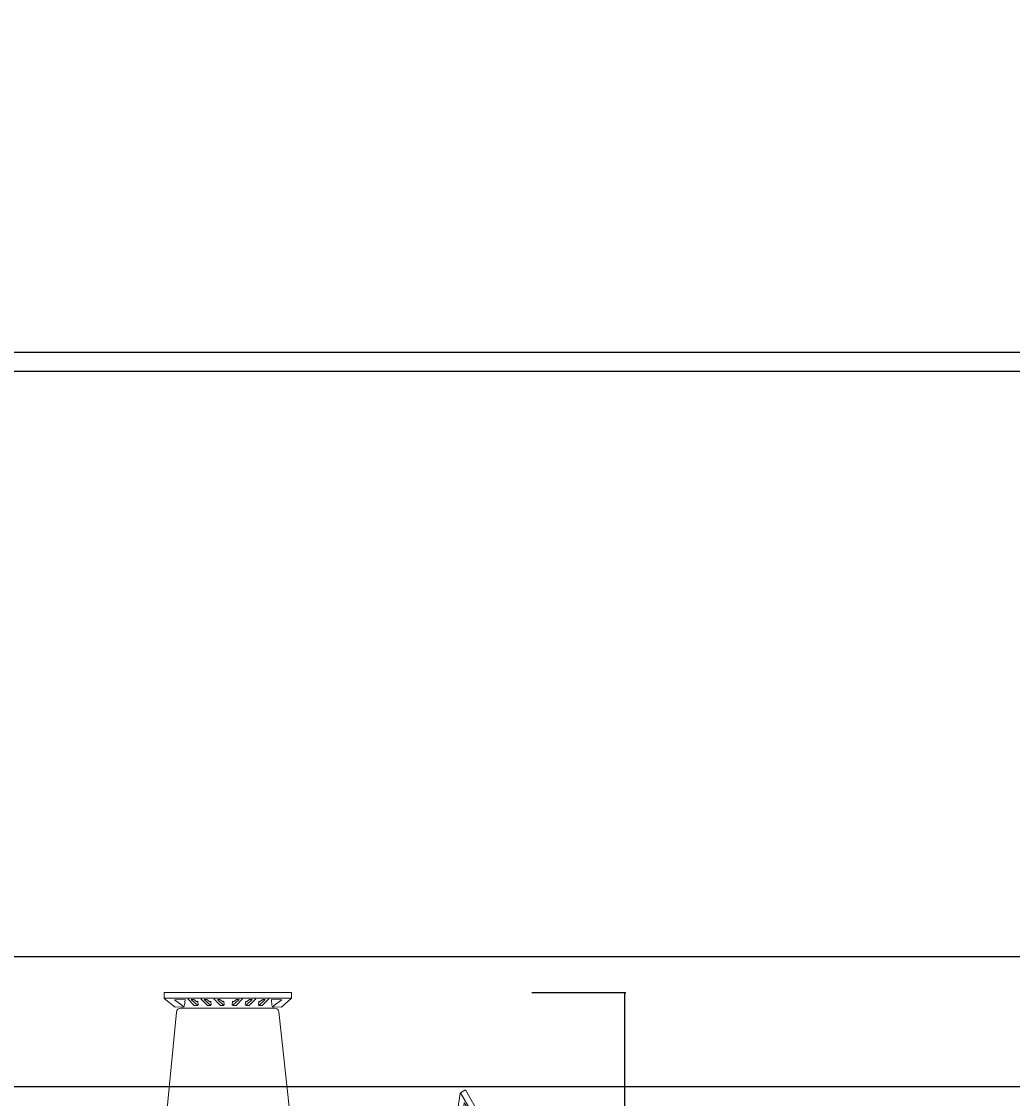
# Model space of a CAD drawing. Units: inches. Extents: x 1865 to 2541, y 1997 to 2759.
# Tile 9 of 11: x 2200 to 2342, y 2405 to 2560. Entities that reach past the tile are written whole.
import ezdxf

# ---------------------------------------------------------------- set-up
doc = ezdxf.new("R2010")
doc.units = ezdxf.units.IN
doc.layers.add('A-ANNO-DIMS', color=2, linetype='Continuous', lineweight=18)
doc.layers.add('DINING TABLE', color=120, linetype='Continuous', lineweight=13)
doc.styles.get("Standard").update_dxf_attribs({"font": 'arial.ttf'})
doc.dimstyles.get("Standard").update_dxf_attribs({"dimtxt": 0.18, "dimasz": 0.18, "dimexe": 0.18, "dimexo": 0.0625, "dimgap": 0.09, "dimtad": 0, "dimtih": 1, "dimtoh": 1, "dimdec": 4, "dimzin": 0, "dimdsep": 46, "dimtxsty": 'Standard', "dimcen": 0.09, "dimadec": 0, "dimazin": 0, "dimtfac": 1, "dimtdec": 4, "dimtofl": 0, "dimtmove": 0, "dimatfit": 3, "dimfxl": 1, "dimtolj": 1, "dimtzin": 0, "dimarcsym": 0})

# ---------------------------------------------------------------- blocks, each defined once
blk = doc.blocks.new('A$C45501D90')
for p, q in [((-242.2, 1133.5), (224, 1133.5)), ((-242.2, 1112.8), (-242.2, 1133.5)), ((224, 1112.8), (-242.2, 1112.8)), ((-242.2, 1111.2), (-202.3, 1079.2)), ((-203.9, 1106.4), (-165.6, 1108)), ((-168.8, 1080.8), (-203.9, 1106.4)), ((-165.6, 1108), (-167.2, 1085.6)), ((-156, 1109.6), (-132, 1085.6)), ((-119.3, 1085.6), (-143.2, 1108)), ((-143.2, 1108), (-133.6, 1108)), ((-133.6, 1108), (-122.5, 1098.4)), ((-108.1, 1109.6), (-84.1, 1085.6)), ((-71.4, 1085.6), (-95.3, 1108)), ((-95.3, 1108), (-85.7, 1108)), ((-85.7, 1108), (-74.6, 1098.4)), ((-60.2, 1109.6), (-36.2, 1085.6)), ((-23.5, 1085.6), (-47.4, 1108)), ((-47.4, 1108), (-37.8, 1108)), ((-37.8, 1108), (-26.7, 1098.4)), ((8.5, 1085.6), (32.4, 1108)), ((22.8, 1108), (11.6, 1098.4)), ((45.2, 1109.6), (21.2, 1085.6)), ((32.4, 1108), (22.8, 1108)), ((56.3, 1085.6), (80.3, 1108)), ((70.7, 1108), (59.5, 1098.4)), ((93.1, 1109.6), (69.1, 1085.6)), ((80.3, 1108), (70.7, 1108)), ((104.2, 1085.6), (128.2, 1108)), ((118.6, 1108), (107.4, 1098.4)), ((141, 1109.6), (117, 1085.6)), ((128.2, 1108), (118.6, 1108)), ((188.9, 1106.4), (150.5, 1108)), ((150.5, 1108), (152.1, 1085.6)), ((153.7, 1080.8), (188.9, 1106.4)), ((224, 1112.8), (187.3, 1079.2)), ((224, 1133.5), (224, 1112.8)), ((-202.3, 1079.2), (-168.8, 1080.8)), ((161.8, 1076.1), (-181.4, 1076.1)), ((-132, 1085.6), (-119.3, 1085.6)), ((-122.5, 1098.4), (-119.3, 1101.6)), ((-119.3, 1101.6), (-117.7, 1087.2)), ((-84.1, 1085.6), (-71.4, 1085.6)), ((-74.6, 1098.4), (-71.4, 1101.6)), ((-71.4, 1101.6), (-69.8, 1087.2)), ((-36.2, 1085.6), (-23.5, 1085.6)), ((-26.7, 1098.4), (-23.5, 1101.6)), ((-23.5, 1101.6), (-21.9, 1087.2)), ((8.5, 1101.6), (6.9, 1087.2)), ((11.6, 1098.4), (8.5, 1101.6)), ((21.2, 1085.6), (8.5, 1085.6)), ((56.3, 1101.6), (54.8, 1087.2)), ((59.5, 1098.4), (56.3, 1101.6)), ((69.1, 1085.6), (56.3, 1085.6)), ((104.2, 1101.6), (102.6, 1087.2)), ((107.4, 1098.4), (104.2, 1101.6)), ((117, 1085.6), (104.2, 1085.6)), ((187.3, 1079.2), (153.7, 1080.8)), ((-197.3, 1061.6), (-238.9, 627.6)), ((225.2, 627.8), (177.6, 1061.8)), ((-1102.7, 357), (-869.7, 760.7)), ((-851.7, 750.4), (-1084.8, 346.6)), ((-869.7, 760.7), (-851.7, 750.4)), ((-848.7, 752.3), (-841, 701.8)), ((841.2, 765.3), (833.5, 714.8)), ((842.6, 766.1), (860.5, 776.5)), ((1075.7, 362.4), (842.6, 766.1)), ((860.5, 776.5), (1093.6, 372.8)), ((-863.7, 716.7), (-884.3, 684.4)), ((-859.2, 673.6), (-863.7, 716.7)), ((833.5, 714.8), (851.7, 686.6)), ((851.7, 686.6), (856.2, 729.8)), ((856.2, 729.8), (876.7, 697.4)), ((-851, 678.1), (-1022.6, 380.9)), ((-890.4, 676.9), (-881.7, 644.2)), ((-884.3, 684.4), (-864.1, 674.6)), ((-841, 701.8), (-859.2, 673.6)), ((-431.1, 509), (-830.8, 684.8)), ((820.7, 701.7), (424.1, 520.7)), ((1012.8, 397.9), (841.2, 695.1)), ((876.7, 697.4), (856.6, 687.6)), ((882.9, 689.9), (874.2, 657.2)), ((880.6, 646.1), (887.9, 678)), ((887.9, 678), (892.7, 669.7)), ((-914.4, 635.4), (-905.6, 602.7)), ((-897.5, 642.2), (-901.9, 641.1)), ((-901.9, 641.1), (-890.2, 632.5)), ((-895.4, 665), (-900.2, 656.7)), ((-900.2, 656.7), (-897.5, 642.2)), ((-888.1, 633.1), (-895.4, 665)), ((-881.7, 644.2), (-888.1, 633.1)), ((874.2, 657.2), (880.6, 646.1)), ((894.4, 654.1), (882.7, 645.5)), ((892.7, 669.7), (890, 655.2)), ((890, 655.2), (894.4, 654.1)), ((906.9, 648.4), (898.1, 615.7)), ((904.5, 604.6), (911.9, 636.5)), ((911.9, 636.5), (916.7, 628.2)), ((-938.3, 593.9), (-929.6, 561.2)), ((-921.5, 600.8), (-925.8, 599.6)), ((-925.8, 599.6), (-914.2, 591)), ((-919.4, 623.5), (-924.2, 615.2)), ((-924.2, 615.2), (-921.5, 600.8)), ((-912, 591.6), (-919.4, 623.5)), ((-905.6, 602.7), (-912, 591.6)), ((-223, 610.1), (209.4, 610.1)), ((898.1, 615.7), (904.5, 604.6)), ((918.3, 612.6), (906.7, 604)), ((916.7, 628.2), (914, 613.8)), ((914, 613.8), (918.3, 612.6)), ((930.8, 606.9), (922.1, 574.2)), ((928.4, 563.1), (935.8, 595.1)), ((935.8, 595.1), (940.6, 586.8)), ((-945.4, 559.3), (-949.8, 558.1)), ((-949.8, 558.1), (-938.1, 549.6)), ((-943.3, 582), (-948.1, 573.8)), ((-948.1, 573.8), (-945.4, 559.3)), ((-936, 550.1), (-943.3, 582)), ((-929.6, 561.2), (-936, 550.1)), ((922.1, 574.2), (928.4, 563.1)), ((942.3, 571.1), (930.6, 562.6)), ((940.6, 586.8), (937.9, 572.3)), ((937.9, 572.3), (942.3, 571.1)), ((-951.9, 522.5), (-983.2, 512.9)), ((-983.2, 512.9), (-978.5, 521.2)), ((-978.5, 521.2), (-964.6, 526.1)), ((-964.6, 526.1), (-965.7, 530.5)), ((-965.7, 530.5), (-952.5, 524.7)), ((-958.3, 511.4), (-951.9, 522.5)), ((950.8, 524.4), (944.4, 535.5)), ((944.4, 535.5), (975.7, 525.9)), ((958.2, 543.5), (945, 537.7)), ((983.5, 515.7), (950.8, 524.4)), ((957.1, 539.1), (958.2, 543.5)), ((970.9, 534.2), (957.1, 539.1)), ((975.7, 525.9), (970.9, 534.2)), ((-975.9, 481), (-1007.2, 471.4)), ((-1007.2, 471.4), (-1002.4, 479.7)), ((-1002.4, 479.7), (-988.5, 484.6)), ((-991, 502.7), (-958.3, 511.4)), ((-988.5, 484.6), (-989.7, 489)), ((-989.7, 489), (-976.5, 483.2)), ((-982.3, 469.9), (-975.9, 481)), ((-639.9, 111.9), (-423.7, 486.4)), ((-5.6, 508.7, 90.8), (0.4, 508.7, 90.8)), ((-5.6, 317.7, 90.8), (-5.6, 508.7, 90.8)), ((0.4, 508.7, 90.8), (0.4, 317.7, 90.8)), ((5.8, 317.7, 90.8), (5.8, 508.7, 90.8)), ((5.8, 508.7, 90.8), (11.8, 508.7, 90.8)), ((11.8, 508.7, 90.8), (11.8, 317.7, 90.8)), ((416.9, 498.2), (633.1, 123.7)), ((968.4, 494), (999.7, 484.4)), ((974.7, 483), (968.4, 494)), ((982.2, 502), (968.9, 496.2)), ((1007.4, 474.2), (974.7, 483)), ((981, 497.6), (982.2, 502)), ((994.9, 492.7), (981, 497.6)), ((999.7, 484.4), (994.9, 492.7)), ((-999.8, 439.5), (-1031.1, 430)), ((-1031.1, 430), (-1026.3, 438.3)), ((-1026.3, 438.3), (-1012.5, 443.1)), ((-1015, 461.2), (-982.3, 469.9)), ((-1012.5, 443.1), (-1013.6, 447.5)), ((-1013.6, 447.5), (-1000.4, 441.7)), ((-1006.2, 428.5), (-999.8, 439.5)), ((998.7, 441.5), (992.3, 452.5)), ((992.3, 452.5), (1023.6, 443)), ((1006.1, 460.5), (992.9, 454.7)), ((1031.4, 432.7), (998.7, 441.5)), ((1005, 456.2), (1006.1, 460.5)), ((1018.8, 451.3), (1005, 456.2)), ((1023.6, 443), (1018.8, 451.3)), ((-1060.1, 376.6), (-1042.3, 410.6)), ((-1020.4, 394.3), (-1060.1, 376.6)), ((-1042.3, 410.6), (-1023.8, 398.1)), ((-1038.9, 419.7), (-1006.2, 428.5)), ((-1035.8, 364.4), (-1020.4, 394.3)), ((1028.3, 377.5), (1012.9, 407.3)), ((1012.9, 407.3), (1052.6, 389.6)), ((1034.8, 423.6), (1016.3, 411.1)), ((1052.6, 389.6), (1034.8, 423.6)), ((-1084.8, 346.6), (-1102.7, 357)), ((-1083.4, 345.8), (-1035.8, 364.4)), ((-1018, 360), (-663, 106.9)), ((656.3, 118.9), (1008.4, 377.1)), ((1075.9, 358.8), (1028.3, 377.5)), ((1093.6, 372.8), (1075.7, 362.4)), ((-22.3, 329.1, 90.8), (-22.3, 344.6, 90.8)), ((-22.3, 344.6, 90.8), (-5.6, 344.6, 90.8)), ((-5.6, 329.1, 90.8), (-22.3, 329.1, 90.8)), ((0.4, 317.7, 90.8), (-5.6, 317.7, 90.8)), ((0.4, 344.6, 90.8), (5.8, 344.6, 90.8)), ((5.8, 329.1, 90.8), (0.4, 329.1, 90.8)), ((11.8, 317.7, 90.8), (5.8, 317.7, 90.8)), ((11.8, 344.6, 90.8), (27.3, 344.6, 90.8)), ((27.3, 329.1, 90.8), (11.8, 329.1, 90.8)), ((27.3, 344.6, 90.8), (27.3, 329.1, 90.8)), ((-430.6, 275.2, 90.8), (-427.6, 280.3, 90.8)), ((-427.6, 280.3, 90.8), (-262.3, 184.9, 90.8)), ((-175.3, 276.1, 90.8), (-104.8, 293.2, 90.8)), ((-103.3, 252.4, 90.8), (-175.3, 276.1, 90.8)), ((-104.8, 293.2, 90.8), (-85.5, 278.4, 90.8)), ((-85.5, 278.4, 90.8), (-52.1, 293.9, 90.8)), ((9.5, 276.1, 90.8), (-59.5, 246.5, 90.8)), ((-52.1, 293.9, 90.8), (9.5, 276.1, 90.8)), ((134.3, 288, 90.8), (184.3, 235.5, 90.8)), ((149.7, 213.9, 90.8), (134.3, 288, 90.8)), ((-436.3, 265.3, 90.8), (-433.3, 270.5, 90.8)), ((-270.9, 169.9, 90.8), (-436.3, 265.3, 90.8)), ((-433.3, 270.5, 90.8), (-267.9, 175, 90.8)), ((-265.2, 179.7, 90.8), (-430.6, 275.2, 90.8)), ((-59.5, 246.5, 90.8), (-103.3, 252.4, 90.8)), ((255.2, 161.9, 90.8), (420.6, 257.3, 90.8)), ((423.5, 252.2, 90.8), (258.2, 156.7, 90.8)), ((260.9, 152, 90.8), (426.2, 247.5, 90.8)), ((429.2, 242.3, 90.8), (263.8, 146.9, 90.8)), ((420.6, 257.3, 90.8), (423.5, 252.2, 90.8)), ((426.2, 247.5, 90.8), (429.2, 242.3, 90.8)), ((-285.5, 198.3, 90.8), (-277.8, 211.7, 90.8)), ((-277.8, 211.7, 90.8), (-264.3, 204, 90.8)), ((-264.3, 204, 90.8), (-272.1, 190.5, 90.8)), ((166.5, 173, 90.8), (149.7, 213.9, 90.8)), ((184.3, 235.5, 90.8), (181.1, 211.4, 90.8)), ((181.1, 211.4, 90.8), (211.3, 190.3, 90.8)), ((-302.5, 168.8, 90.8), (-294.2, 183.3, 90.8)), ((-289.1, 161.1, 90.8), (-302.5, 168.8, 90.8)), ((-291.2, 188.5, 90.8), (-288.5, 193.1, 90.8)), ((-280.7, 175.5, 90.8), (-289.1, 161.1, 90.8)), ((-275.1, 185.4, 90.8), (-277.8, 180.7, 90.8)), ((-273.6, 117.6, 90.8), (-227.4, 162.1, 90.8)), ((-267.9, 175, 90.8), (-270.9, 169.9, 90.8)), ((-262.3, 184.9, 90.8), (-265.2, 179.7, 90.8)), ((-227.4, 162.1, 90.8), (-236.2, 87.5, 90.8)), ((226.7, 128.1, 90.8), (166.5, 173, 90.8)), ((211.3, 190.3, 90.8), (226.7, 128.1, 90.8)), ((258.2, 156.7, 90.8), (255.2, 161.9, 90.8)), ((256.6, 182, 90.8), (270.1, 189.8, 90.8)), ((265, 167.5, 90.8), (256.6, 182, 90.8)), ((270.7, 157.7, 90.8), (268, 162.4, 90.8)), ((270.1, 189.8, 90.8), (278.4, 175.3, 90.8)), ((281.4, 170.1, 90.8), (284.1, 165.5, 90.8)), ((287.1, 160.3, 90.8), (294.9, 146.8, 90.8)), ((263.8, 146.9, 90.8), (260.9, 152, 90.8)), ((281.4, 139.1, 90.8), (273.7, 152.5, 90.8)), ((294.9, 146.8, 90.8), (281.4, 139.1, 90.8)), ((-299.3, 71.7, 90.8), (-276.8, 80.9, 90.8)), ((-276.8, 80.9, 90.8), (-273.6, 117.6, 90.8)), ((-236.2, 87.5, 90.8), (-263.2, 52.5, 90.8)), ((-319.8, 2.1, 90.8), (-299.3, 71.7, 90.8)), ((-263.2, 52.5, 90.8), (-319.8, 2.1, 90.8)), ((242.9, -24.6, 90.8), (299.4, 25.9, 90.8)), ((299.4, 25.9, 90.8), (278.9, -43.7, 90.8)), ((215.8, -59.5, 90.8), (242.9, -24.6, 90.8)), ((207, -134.1, 90.8), (215.8, -59.5, 90.8)), ((256.4, -53, 90.8), (253.2, -89.7, 90.8)), ((278.9, -43.7, 90.8), (256.4, -53, 90.8)), ((-315.2, -118.9, 90.8), (-301.8, -111.1, 90.8)), ((-301.8, -111.1, 90.8), (-294, -124.6, 90.8)), ((-247, -100.1, 90.8), (-186.8, -145, 90.8)), ((-231.7, -162.3, 90.8), (-247, -100.1, 90.8)), ((253.2, -89.7, 90.8), (207, -134.1, 90.8)), ((639.9, -111.9), (423.7, -486.4)), ((1018, -360), (663, -106.9)), ((-656.3, -118.9), (-1008.4, -377.1)), ((-416.9, -498.2), (-633.1, -123.7)), ((-449.6, -214.4, 90.8), (-284.2, -118.9, 90.8)), ((-281.2, -124.1, 90.8), (-446.6, -219.5, 90.8)), ((-443.9, -224.2, 90.8), (-278.5, -128.7, 90.8)), ((-275.5, -133.9, 90.8), (-440.9, -229.4, 90.8)), ((-307.5, -132.3, 90.8), (-315.2, -118.9, 90.8)), ((-301.8, -142.1, 90.8), (-304.5, -137.5, 90.8)), ((-290.4, -161.8, 90.8), (-298.8, -147.3, 90.8)), ((-291, -129.7, 90.8), (-288.3, -134.4, 90.8)), ((-277, -154, 90.8), (-290.4, -161.8, 90.8)), ((-285.4, -139.5, 90.8), (-277, -154, 90.8)), ((-284.2, -118.9, 90.8), (-281.2, -124.1, 90.8)), ((-278.5, -128.7, 90.8), (-275.5, -133.9, 90.8)), ((-186.8, -145, 90.8), (-170.1, -185.9, 90.8)), ((241.9, -156.9, 90.8), (244.9, -151.7, 90.8)), ((407.3, -252.4, 90.8), (241.9, -156.9, 90.8)), ((244.9, -151.7, 90.8), (410.3, -247.2, 90.8)), ((247.6, -147.1, 90.8), (250.6, -141.9, 90.8)), ((413, -242.5, 90.8), (247.6, -147.1, 90.8)), ((250.6, -141.9, 90.8), (415.9, -237.4, 90.8)), ((254.7, -157.4, 90.8), (257.4, -152.7, 90.8)), ((260.4, -147.6, 90.8), (268.7, -133.1, 90.8)), ((268.7, -133.1, 90.8), (282.2, -140.8, 90.8)), ((282.2, -140.8, 90.8), (273.8, -155.3, 90.8)), ((-201.5, -183.4, 90.8), (-231.7, -162.3, 90.8)), ((-204.7, -207.6, 90.8), (-201.5, -183.4, 90.8)), ((-170.1, -185.9, 90.8), (-154.7, -260.1, 90.8)), ((244, -176, 90.8), (251.7, -162.5, 90.8)), ((257.4, -183.7, 90.8), (244, -176, 90.8)), ((265.2, -170.3, 90.8), (257.4, -183.7, 90.8)), ((270.8, -160.5, 90.8), (268.1, -165.1, 90.8)), ((-446.6, -219.5, 90.8), (-449.6, -214.4, 90.8)), ((-440.9, -229.4, 90.8), (-443.9, -224.2, 90.8)), ((-154.7, -260.1, 90.8), (-204.7, -207.6, 90.8)), ((-29.8, -248.2, 90.8), (39.2, -218.5, 90.8)), ((39.2, -218.5, 90.8), (83, -224.4, 90.8)), ((83, -224.4, 90.8), (154.9, -248.2, 90.8)), ((31.8, -266, 90.8), (-29.8, -248.2, 90.8)), ((65.2, -250.4, 90.8), (31.8, -266, 90.8)), ((84.4, -265.2, 90.8), (65.2, -250.4, 90.8)), ((154.9, -248.2, 90.8), (84.4, -265.2, 90.8)), ((410.3, -247.2, 90.8), (407.3, -252.4, 90.8)), ((415.9, -237.4, 90.8), (413, -242.5, 90.8)), ((-47.6, -316.6, 90.8), (-47.6, -301.1, 90.8)), ((-47.6, -301.1, 90.8), (-32.1, -301.1, 90.8)), ((-32.1, -480.7, 90.8), (-32.1, -289.8, 90.8)), ((-32.1, -289.8, 90.8), (-26.1, -289.8, 90.8)), ((-26.1, -289.8, 90.8), (-26.1, -480.7, 90.8)), ((-26.1, -301.1, 90.8), (-20.8, -301.1, 90.8)), ((-20.8, -480.7, 90.8), (-20.8, -289.8, 90.8)), ((-20.8, -289.8, 90.8), (-14.8, -289.8, 90.8)), ((-14.8, -289.8, 90.8), (-14.8, -480.7, 90.8)), ((-14.8, -301.1, 90.8), (1.9, -301.1, 90.8)), ((1.9, -301.1, 90.8), (1.9, -316.6, 90.8)), ((-32.1, -316.6, 90.8), (-47.6, -316.6, 90.8)), ((-20.8, -316.6, 90.8), (-26.1, -316.6, 90.8)), ((1.9, -316.6, 90.8), (-14.8, -316.6, 90.8)), ((851.7, -750.4), (1084.8, -346.6)), ((1083.4, -345.8), (1035.8, -364.4)), ((1084.8, -346.6), (1102.7, -357)), ((-1093.6, -372.8), (-1075.7, -362.4)), ((-860.5, -776.5), (-1093.6, -372.8)), ((-1075.9, -358.8), (-1028.3, -377.5)), ((-1075.7, -362.4), (-842.6, -766.1)), ((-1052.6, -389.6), (-1034.8, -423.6)), ((-1012.9, -407.3), (-1052.6, -389.6)), ((-1028.3, -377.5), (-1012.9, -407.3)), ((851, -678.1), (1022.6, -380.9)), ((1102.7, -357), (869.7, -760.7)), ((1035.8, -364.4), (1020.4, -394.3)), ((1020.4, -394.3), (1060.1, -376.6)), ((1060.1, -376.6), (1042.3, -410.6)), ((-1034.8, -423.6), (-1016.3, -411.1)), ((-1031.4, -432.7), (-998.7, -441.5)), ((-1012.8, -397.9), (-841.2, -695.1)), ((1006.2, -428.5), (999.8, -439.5)), ((999.8, -439.5), (1031.1, -430)), ((1038.9, -419.7), (1006.2, -428.5)), ((1042.3, -410.6), (1023.8, -398.1)), ((1031.1, -430), (1026.3, -438.3)), ((-1023.6, -443), (-1018.8, -451.3)), ((-992.3, -452.5), (-1023.6, -443)), ((-1018.8, -451.3), (-1005, -456.2)), ((-1006.1, -460.5), (-992.9, -454.7)), ((-1005, -456.2), (-1006.1, -460.5)), ((-998.7, -441.5), (-992.3, -452.5)), ((982.3, -469.9), (975.9, -481)), ((975.9, -481), (1007.2, -471.4)), ((1015, -461.2), (982.3, -469.9)), ((1013.6, -447.5), (1000.4, -441.7)), ((1007.2, -471.4), (1002.4, -479.7)), ((1026.3, -438.3), (1012.5, -443.1)), ((1012.5, -443.1), (1013.6, -447.5)), ((-1007.4, -474.2), (-974.7, -483)), ((-968.4, -494), (-999.7, -484.4)), ((-999.7, -484.4), (-994.9, -492.7)), ((-994.9, -492.7), (-981, -497.6)), ((-982.2, -502), (-968.9, -496.2)), ((-981, -497.6), (-982.2, -502)), ((-974.7, -483), (-968.4, -494)), ((-26.1, -480.7, 90.8), (-32.1, -480.7, 90.8)), ((-14.8, -480.7, 90.8), (-20.8, -480.7, 90.8)), ((431.1, -509), (830.8, -684.8)), ((958.3, -511.4), (951.9, -522.5)), ((991, -502.7), (958.3, -511.4)), ((989.7, -489), (976.5, -483.2)), ((1002.4, -479.7), (988.5, -484.6)), ((988.5, -484.6), (989.7, -489)), ((-983.5, -515.7), (-950.8, -524.4)), ((-944.4, -535.5), (-975.7, -525.9)), ((-975.7, -525.9), (-970.9, -534.2)), ((-970.9, -534.2), (-957.1, -539.1)), ((-958.2, -543.5), (-945, -537.7)), ((-957.1, -539.1), (-958.2, -543.5)), ((-950.8, -524.4), (-944.4, -535.5)), ((-820.7, -701.7), (-424.1, -520.7)), ((929.6, -561.2), (936, -550.1)), ((936, -550.1), (943.3, -582)), ((949.8, -558.1), (938.1, -549.6)), ((951.9, -522.5), (983.2, -512.9)), ((965.7, -530.5), (952.5, -524.7)), ((978.5, -521.2), (964.6, -526.1)), ((964.6, -526.1), (965.7, -530.5)), ((983.2, -512.9), (978.5, -521.2)), ((-942.3, -571.1), (-930.6, -562.6)), ((-937.9, -572.3), (-942.3, -571.1)), ((-940.6, -586.8), (-937.9, -572.3)), ((-935.8, -595.1), (-940.6, -586.8)), ((-928.4, -563.1), (-935.8, -595.1)), ((-930.8, -606.9), (-922.1, -574.2)), ((-922.1, -574.2), (-928.4, -563.1)), ((925.8, -599.6), (914.2, -591)), ((938.3, -593.9), (929.6, -561.2)), ((943.3, -582), (948.1, -573.8)), ((945.4, -559.3), (949.8, -558.1)), ((948.1, -573.8), (945.4, -559.3)), ((-918.3, -612.6), (-906.7, -604)), ((-914, -613.8), (-918.3, -612.6)), ((-916.7, -628.2), (-914, -613.8)), ((-911.9, -636.5), (-916.7, -628.2)), ((-904.5, -604.6), (-911.9, -636.5)), ((-906.9, -648.4), (-898.1, -615.7)), ((-898.1, -615.7), (-904.5, -604.6)), ((-229.3, -629.3), (-181.8, -1063.3)), ((-225.2, -627.8), (-177.6, -1061.8)), ((218.9, -611.6), (-213.5, -611.6)), ((223, -610.1), (-209.4, -610.1)), ((193.2, -1063.1), (234.8, -629.1)), ((197.3, -1061.6), (238.9, -627.6)), ((905.6, -602.7), (912, -591.6)), ((914.4, -635.4), (905.6, -602.7)), ((912, -591.6), (919.4, -623.5)), ((919.4, -623.5), (924.2, -615.2)), ((921.5, -600.8), (925.8, -599.6)), ((924.2, -615.2), (921.5, -600.8)), ((-894.4, -654.1), (-882.7, -645.5)), ((-890, -655.2), (-894.4, -654.1)), ((-892.7, -669.7), (-890, -655.2)), ((-887.9, -678), (-892.7, -669.7)), ((-880.6, -646.1), (-887.9, -678)), ((-882.9, -689.9), (-874.2, -657.2)), ((-874.2, -657.2), (-880.6, -646.1)), ((881.7, -644.2), (888.1, -633.1)), ((890.4, -676.9), (881.7, -644.2)), ((888.1, -633.1), (895.4, -665)), ((901.9, -641.1), (890.2, -632.5)), ((895.4, -665), (900.2, -656.7)), ((897.5, -642.2), (901.9, -641.1)), ((900.2, -656.7), (897.5, -642.2)), ((-876.7, -697.4), (-856.6, -687.6)), ((-856.2, -729.8), (-876.7, -697.4)), ((-851.7, -686.6), (-856.2, -729.8)), ((-833.5, -714.8), (-851.7, -686.6)), ((841, -701.8), (859.2, -673.6)), ((848.7, -752.3), (841, -701.8)), ((859.2, -673.6), (863.7, -716.7)), ((863.7, -716.7), (884.3, -684.4)), ((884.3, -684.4), (864.1, -674.6)), ((-841.2, -765.3), (-833.5, -714.8)), ((-842.6, -766.1), (-860.5, -776.5)), ((869.7, -760.7), (851.7, -750.4)), ((-231.3, -1112.7), (-191.4, -1080.8)), ((-227.2, -1111.2), (-187.3, -1079.2)), ((-157.9, -1082.4), (-193, -1107.9)), ((-191.4, -1080.8), (-157.9, -1082.4)), ((-153.7, -1080.8), (-188.9, -1106.4)), ((-187.3, -1079.2), (-153.7, -1080.8)), ((-165.9, -1077.6), (177.3, -1077.6)), ((-161.8, -1076.1), (181.4, -1076.1)), ((-154.7, -1109.5), (-156.3, -1087.1)), ((-150.5, -1108), (-152.1, -1085.6)), ((-145.1, -1111.1), (-121.1, -1087.1)), ((-141, -1109.6), (-117, -1085.6)), ((-108.4, -1087.1), (-132.3, -1109.5)), ((-104.2, -1085.6), (-128.2, -1108)), ((-122.7, -1109.5), (-111.6, -1099.9)), ((-121.1, -1087.1), (-108.4, -1087.1)), ((-118.6, -1108), (-107.4, -1098.4)), ((-117, -1085.6), (-104.2, -1085.6)), ((-111.6, -1099.9), (-108.4, -1103.1)), ((-108.4, -1103.1), (-106.8, -1088.7)), ((-107.4, -1098.4), (-104.2, -1101.6)), ((-104.2, -1101.6), (-102.6, -1087.2)), ((-97.2, -1111.1), (-73.2, -1087.1)), ((-93.1, -1109.6), (-69.1, -1085.6)), ((-60.5, -1087.1), (-84.4, -1109.5)), ((-56.3, -1085.6), (-80.3, -1108)), ((-74.8, -1109.5), (-63.7, -1099.9)), ((-73.2, -1087.1), (-60.5, -1087.1)), ((-70.7, -1108), (-59.5, -1098.4)), ((-69.1, -1085.6), (-56.3, -1085.6)), ((-63.7, -1099.9), (-60.5, -1103.1)), ((-60.5, -1103.1), (-58.9, -1088.7)), ((-59.5, -1098.4), (-56.3, -1101.6)), ((-56.3, -1101.6), (-54.8, -1087.2)), ((-49.3, -1111.1), (-25.3, -1087.1)), ((-45.2, -1109.6), (-21.2, -1085.6)), ((-12.6, -1087.1), (-36.5, -1109.5)), ((-8.5, -1085.6), (-32.4, -1108)), ((-26.9, -1109.5), (-15.8, -1099.9)), ((-25.3, -1087.1), (-12.6, -1087.1)), ((-22.8, -1108), (-11.6, -1098.4)), ((-21.2, -1085.6), (-8.5, -1085.6)), ((-15.8, -1099.9), (-12.6, -1103.1)), ((-12.6, -1103.1), (-11, -1088.7)), ((-11.6, -1098.4), (-8.5, -1101.6)), ((-8.5, -1101.6), (-6.9, -1087.2)), ((19.4, -1103.1), (17.8, -1088.7)), ((19.4, -1087.1), (43.3, -1109.5)), ((32.1, -1087.1), (19.4, -1087.1)), ((22.6, -1099.9), (19.4, -1103.1)), ((23.5, -1101.6), (21.9, -1087.2)), ((33.7, -1109.5), (22.6, -1099.9)), ((23.5, -1085.6), (47.4, -1108)), ((36.2, -1085.6), (23.5, -1085.6)), ((26.7, -1098.4), (23.5, -1101.6)), ((37.8, -1108), (26.7, -1098.4)), ((56.1, -1111.1), (32.1, -1087.1)), ((60.2, -1109.6), (36.2, -1085.6)), ((67.3, -1103.1), (65.7, -1088.7)), ((67.3, -1087.1), (91.2, -1109.5)), ((80, -1087.1), (67.3, -1087.1)), ((70.4, -1099.9), (67.3, -1103.1)), ((71.4, -1101.6), (69.8, -1087.2)), ((81.6, -1109.5), (70.4, -1099.9)), ((71.4, -1085.6), (95.3, -1108)), ((84.1, -1085.6), (71.4, -1085.6)), ((74.6, -1098.4), (71.4, -1101.6)), ((85.7, -1108), (74.6, -1098.4)), ((104, -1111.1), (80, -1087.1)), ((108.1, -1109.6), (84.1, -1085.6)), ((115.1, -1103.1), (113.6, -1088.7)), ((115.1, -1087.1), (139.1, -1109.5)), ((127.9, -1087.1), (115.1, -1087.1)), ((118.3, -1099.9), (115.1, -1103.1)), ((119.3, -1101.6), (117.7, -1087.2)), ((129.5, -1109.5), (118.3, -1099.9)), ((119.3, -1085.6), (143.2, -1108)), ((132, -1085.6), (119.3, -1085.6)), ((122.5, -1098.4), (119.3, -1101.6)), ((133.6, -1108), (122.5, -1098.4)), ((151.9, -1111.1), (127.9, -1087.1)), ((156, -1109.6), (132, -1085.6)), ((161.4, -1109.5), (163, -1087.1)), ((198.2, -1080.8), (164.6, -1082.4)), ((164.6, -1082.4), (199.8, -1107.9)), ((165.6, -1108), (167.2, -1085.6)), ((202.3, -1079.2), (168.8, -1080.8)), ((168.8, -1080.8), (203.9, -1106.4)), ((238.1, -1112.7), (198.2, -1080.8)), ((242.2, -1111.2), (202.3, -1079.2)), ((-228.1, -1114.3), (238.1, -1114.3)), ((-228.1, -1135), (-228.1, -1114.3)), ((238.1, -1135), (-228.1, -1135)), ((-224, -1112.8), (242.2, -1112.8)), ((-224, -1133.5), (-224, -1112.8)), ((242.2, -1133.5), (-224, -1133.5)), ((-193, -1107.9), (-154.7, -1109.5)), ((-188.9, -1106.4), (-150.5, -1108)), ((-132.3, -1109.5), (-122.7, -1109.5)), ((-128.2, -1108), (-118.6, -1108)), ((-84.4, -1109.5), (-74.8, -1109.5)), ((-80.3, -1108), (-70.7, -1108)), ((-36.5, -1109.5), (-26.9, -1109.5)), ((-32.4, -1108), (-22.8, -1108)), ((43.3, -1109.5), (33.7, -1109.5)), ((47.4, -1108), (37.8, -1108)), ((91.2, -1109.5), (81.6, -1109.5)), ((95.3, -1108), (85.7, -1108)), ((139.1, -1109.5), (129.5, -1109.5)), ((143.2, -1108), (133.6, -1108)), ((199.8, -1107.9), (161.4, -1109.5)), ((203.9, -1106.4), (165.6, -1108)), ((238.1, -1114.3), (238.1, -1135)), ((242.2, -1112.8), (242.2, -1133.5))]:
    blk.add_line(p, q)
for centre, radius in [((0, 0), 537), ((0, 0), 527), ((-94.8, 394.7, 90.8), 61.3), ((96.9, 390, 90.8), 56.9), ((95.5, 390.7, 90.8), 29.4), ((-282.3, 294.7, 90.8), 56.9), ((-283.5, 293.9, 90.8), 29.4), ((277.2, 277.6, 90.8), 61.3), ((-382.1, 131.1, 90.8), 61.3), ((369, 109.3, 90.8), 56.9), ((368.9, 110.8, 90.8), 29.4), ((-389.3, -81.3, 90.8), 56.9), ((-389.2, -82.8, 90.8), 29.4), ((361.8, -103.1, 90.8), 61.3), ((-297.5, -249.6, 90.8), 61.3), ((261.9, -266.7, 90.8), 56.9), ((263.2, -265.9, 90.8), 29.4), ((-117.2, -362, 90.8), 56.9), ((74.4, -366.7, 90.8), 61.3), ((-115.9, -362.7, 90.8), 29.4)]:
    blk.add_circle(centre, radius)
for centre, radius, start, end in [((-181.4, 1060.1), 16, 90, 174.5199), ((161.8, 1060.1), 16, 6.2572, 90), ((-837.2, 670.1), 16, 66.2572, 150), ((827.4, 687.1), 16, 30, 114.5199), ((-223, 626.1), 16, 174.5199, 270), ((209.4, 626.1), 16, 270, 6.2572), ((430.7, 506.2), 16, 114.5199, 210), ((-437.5, 494.4), 16, 330, 66.2572), ((999, 389.9), 16, 306.2572, 30), ((-1008.8, 373), 16, 150, 234.5199), ((-77.3, 270.2, 90.8), 44.6, 25.8558, 153.3359), ((-77.3, 270.2, 90.8), 44.6, 195.9338, 342.9389), ((178.1, 200.3, 90.8), 44.6, 325.8558, 93.3359), ((178.1, 200.3, 90.8), 44.6, 135.9338, 282.9389), ((-265.7, 83.9, 90.8), 44.6, 85.8558, 213.3359), ((646.9, 131.7), 16, 210, 306.2572), ((-653.7, 119.9), 16, 234.5199, 330), ((-265.7, 83.9, 90.8), 44.6, 255.9338, 42.9389), ((245.3, -55.9, 90.8), 44.6, 75.9338, 222.9389), ((245.3, -55.9, 90.8), 44.6, 265.8558, 33.3359), ((-646.9, -131.7), 16, 30, 126.2572), ((653.7, -119.9), 16, 54.5199, 150), ((-198.5, -172.3, 90.8), 44.6, 145.8558, 273.3359), ((-198.5, -172.3, 90.8), 44.6, 315.9338, 102.9389), ((57, -242.2, 90.8), 44.6, 15.9338, 162.9389), ((57, -242.2, 90.8), 44.6, 205.8558, 333.3359), ((-999, -389.9), 16, 126.2572, 210), ((1008.8, -373), 16, 330, 54.5199), ((-430.7, -506.2), 16, 294.5199, 30), ((437.5, -494.4), 16, 150, 246.2572), ((-213.5, -627.6), 16, 90, 186.2572), ((-209.4, -626.1), 16, 90, 186.2572), ((218.9, -627.6), 16, 354.5199, 90), ((223, -626.1), 16, 354.5199, 90), ((-827.4, -687.1), 16, 210, 294.5199), ((837.2, -670.1), 16, 246.2572, 330), ((-165.9, -1061.6), 16, 186.2572, 270), ((-161.8, -1060.1), 16, 186.2572, 270), ((177.3, -1061.6), 16, 270, 354.5199), ((181.4, -1060.1), 16, 270, 354.5199)]:
    blk.add_arc(centre, radius, start, end)
blk = doc.blocks.new('*D38')
at = {"layer": 'A-ANNO-DIMS', "color": 0, "lineweight": -2, "transparency": 16777216}
for p, q in [((2273.08, 2420.54), (2286.59, 2420.54)), ((2286.41, 2420.36), (2286.41, 2376.07)), ((2286.41, 2331.41), (2286.41, 2375.7)), ((2273.08, 2331.23), (2286.59, 2331.23))]:
    blk.add_line(p, q, dxfattribs=at)
at = {"layer": 'A-ANNO-DIMS', "color": 0, "transparency": 16777216}
for points in [[(2286.38, 2420.36), (2286.44, 2420.36), (2286.41, 2420.54)], [(2286.38, 2331.41), (2286.44, 2331.41), (2286.41, 2331.23)]]:
    blk.add_solid(points, dxfattribs=at)
at = {"layer": 'Defpoints', "color": 0, "transparency": 16777216}
for p in [(2273.02, 2420.54), (2286.41, 2420.54), (2273.02, 2331.23)]:
    blk.add_point(p, dxfattribs=at)
at = {"layer": 'A-ANNO-DIMS', "color": 0, "transparency": 16777216, "insert": (2286.41, 2375.89), "char_height": 0.18, "attachment_point": 5}
blk.add_mtext('\\A1;DINING SET 89', dxfattribs=at)
blk = doc.blocks.new('*D41')
at = {"layer": 'A-ANNO-DIMS', "color": 0, "lineweight": -2, "transparency": 16777216}
for p, q in [((2503.31, 2721.45), (2540.92, 2721.45)), ((2540.74, 2721.27), (2540.74, 2378.49)), ((2540.74, 2035.35), (2540.74, 2378.13)), ((2136.19, 2035.17), (2540.92, 2035.17))]:
    blk.add_line(p, q, dxfattribs=at)
at = {"layer": 'A-ANNO-DIMS', "color": 0, "transparency": 16777216}
for points in [[(2540.71, 2721.27), (2540.77, 2721.27), (2540.74, 2721.45)], [(2540.71, 2035.35), (2540.77, 2035.35), (2540.74, 2035.17)]]:
    blk.add_solid(points, dxfattribs=at)
at = {"layer": 'Defpoints', "color": 0, "transparency": 16777216}
for p in [(2503.24, 2721.45), (2136.13, 2035.17), (2540.74, 2035.17)]:
    blk.add_point(p, dxfattribs=at)
at = {"layer": 'A-ANNO-DIMS', "color": 0, "transparency": 16777216, "insert": (2540.74, 2378.31), "char_height": 0.18, "attachment_point": 5}
blk.add_mtext('\\A1;686.3', dxfattribs=at)
blk = doc.blocks.new('*D63')
at = {"layer": 'A-ANNO-DIMS', "color": 0, "lineweight": -2, "transparency": 16777216}
for p, q in [((2404.18, 2563.95), (1865.56, 2563.95)), ((1865.74, 2563.77), (1865.74, 2538.51)), ((1865.74, 2512.9), (1865.74, 2538.15)), ((2404.18, 2512.72), (1865.56, 2512.72))]:
    blk.add_line(p, q, dxfattribs=at)
at = {"layer": 'A-ANNO-DIMS', "color": 0, "transparency": 16777216}
for points in [[(1865.71, 2563.77), (1865.77, 2563.77), (1865.74, 2563.95)], [(1865.71, 2512.9), (1865.77, 2512.9), (1865.74, 2512.72)]]:
    blk.add_solid(points, dxfattribs=at)
at = {"layer": 'Defpoints', "color": 0, "transparency": 16777216}
for p in [(2404.24, 2563.95), (1865.74, 2512.72), (2404.24, 2512.72)]:
    blk.add_point(p, dxfattribs=at)
at = {"layer": 'A-ANNO-DIMS', "color": 0, "transparency": 16777216, "insert": (1865.74, 2538.33), "char_height": 0.18, "attachment_point": 5}
blk.add_mtext('\\A1;51.23', dxfattribs=at)
blk = doc.blocks.new('*D66')
at = {"layer": 'A-ANNO-DIMS', "color": 0, "lineweight": -2, "transparency": 16777216}
for p, q in [((2408.32, 2425.66), (1865.56, 2425.66)), ((1865.74, 2425.48), (1865.74, 2416.48)), ((1865.74, 2407.13), (1865.74, 2416.12)), ((2408.32, 2406.95), (1865.56, 2406.95))]:
    blk.add_line(p, q, dxfattribs=at)
at = {"layer": 'A-ANNO-DIMS', "color": 0, "transparency": 16777216}
for points in [[(1865.71, 2425.48), (1865.77, 2425.48), (1865.74, 2425.66)], [(1865.71, 2407.13), (1865.77, 2407.13), (1865.74, 2406.95)]]:
    blk.add_solid(points, dxfattribs=at)
at = {"layer": 'Defpoints', "color": 0, "transparency": 16777216}
for p in [(2408.38, 2425.66), (1865.74, 2406.95), (2408.38, 2406.95)]:
    blk.add_point(p, dxfattribs=at)
at = {"layer": 'A-ANNO-DIMS', "color": 0, "transparency": 16777216, "insert": (1865.74, 2416.3), "char_height": 0.18, "attachment_point": 5}
blk.add_mtext('\\A1;18.706', dxfattribs=at)
blk = doc.blocks.new('*D67')
at = {"layer": 'A-ANNO-DIMS', "color": 0, "lineweight": -2, "transparency": 16777216}
for p, q in [((2475.89, 2509.99), (1865.56, 2509.99)), ((1865.74, 2509.81), (1865.74, 2468)), ((1865.74, 2425.84), (1865.74, 2467.64)), ((2475.89, 2425.66), (1865.56, 2425.66))]:
    blk.add_line(p, q, dxfattribs=at)
at = {"layer": 'A-ANNO-DIMS', "color": 0, "transparency": 16777216}
for points in [[(1865.71, 2509.81), (1865.77, 2509.81), (1865.74, 2509.99)], [(1865.71, 2425.84), (1865.77, 2425.84), (1865.74, 2425.66)]]:
    blk.add_solid(points, dxfattribs=at)
at = {"layer": 'Defpoints', "color": 0, "transparency": 16777216}
for p in [(1865.74, 2509.99), (2475.95, 2509.99), (2475.95, 2425.66)]:
    blk.add_point(p, dxfattribs=at)
at = {"layer": 'A-ANNO-DIMS', "color": 0, "transparency": 16777216, "insert": (1865.74, 2467.82), "char_height": 0.18, "attachment_point": 5}
blk.add_mtext('\\A1;84.33', dxfattribs=at)

msp = doc.modelspace()

# ---------------------------------------------------------------- block references
at = {"layer": 'DINING TABLE', "xscale": 0.0393700787401575, "yscale": 0.0393700787401575, "zscale": 0.0393700787401575}
msp.add_blockref('A$C45501D90', (2229.6028, 2375.915, -3.5735), dxfattribs=at)

# ---------------------------------------------------------------- dimensions: what is measured, and where the dimension line sits
at = {"layer": 'A-ANNO-DIMS'}
for base, p1, p2, override, picture, middle in [((2540.743, 2035.1708), (2503.243, 2721.4494), (2136.13, 2035.1708), {"dimdec": 1, "dimlfac": 1, "dimrnd": 0, "dimzin": 0, "dimdsep": 46, "dimlunit": 2}, '*D41', (2540.743, 2378.3101)), ((1865.743, 2512.7166), (2404.243, 2563.9494), (2404.243, 2512.7166), {"dimdec": 2, "dimlfac": 1, "dimrnd": 0, "dimzin": 0, "dimdsep": 46, "dimlunit": 2}, '*D63', (1865.743, 2538.333)), ((1865.743, 2509.9875), (2475.9518, 2425.6552), (2475.9518, 2509.9875), {"dimdec": 2, "dimlfac": 1, "dimrnd": 0, "dimzin": 0, "dimdsep": 46, "dimlunit": 2}, '*D67', (1865.743, 2467.8214)), ((1865.743, 2406.9494), (2408.3779, 2425.6552), (2408.3779, 2406.9494), {"dimdec": 3, "dimlfac": 1, "dimrnd": 0, "dimzin": 0, "dimdsep": 46, "dimlunit": 2}, '*D66', (1865.743, 2416.3023))]:
    dim = msp.add_linear_dim(base=base, p1=p1, p2=p2, angle=90, dimstyle='Standard', override=override, dxfattribs=at)
    dim.commit()
    dim.dimension.update_dxf_attribs({"geometry": picture, "text_midpoint": middle})
dim = msp.add_linear_dim(base=(2286.4145, 2420.541), p1=(2273.0177, 2331.2292), p2=(2273.0177, 2420.541), angle=90, text='DINING SET <>', dimstyle='Standard', override={"dimdec": 0, "dimlfac": 1, "dimrnd": 0, "dimzin": 0, "dimdsep": 46, "dimlunit": 2}, dxfattribs=at)
dim.commit()
dim.dimension.update_dxf_attribs({"geometry": '*D38', "text_midpoint": (2286.4145, 2375.8851)})

doc.saveas('drawing.dxf')
